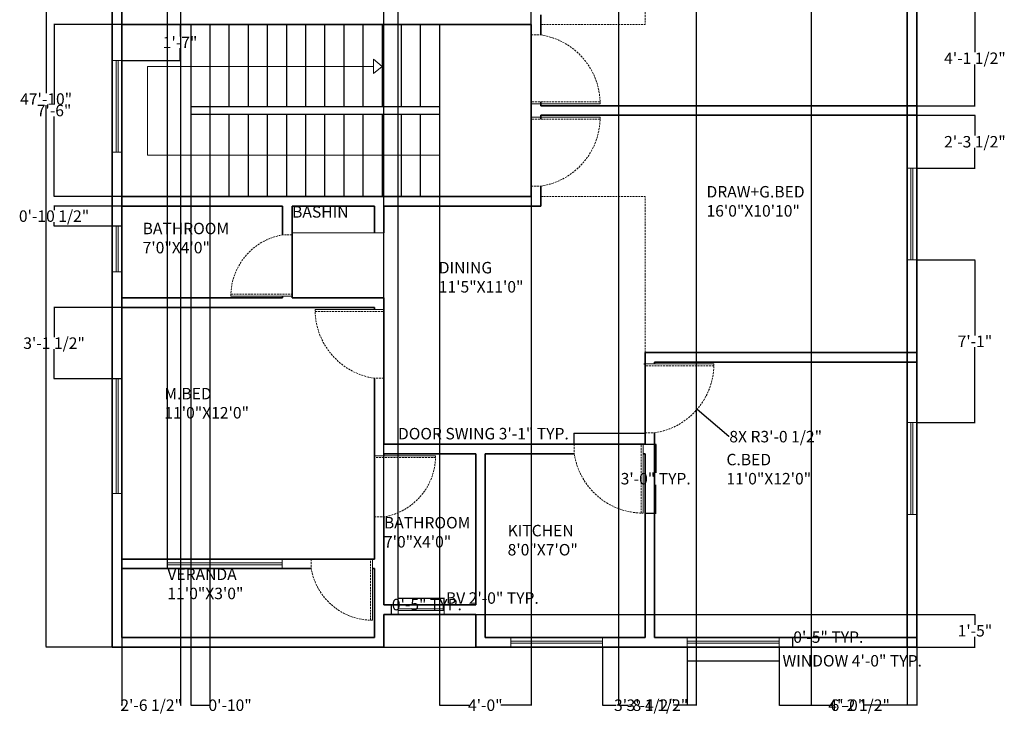
# Model space of a CAD drawing. Units: inches. Extents: x 32162 to 32679, y 109297 to 109949.
# Tile 1 of 2: x 32162 to 32677, y 109297 to 109665. Entities that reach past the tile are written whole.
import ezdxf

# ---------------------------------------------------------------- set-up
doc = ezdxf.new("R2010")
doc.units = ezdxf.units.IN
doc.header["$MEASUREMENT"] = 0
doc.linetypes.add('DASHEDX2', pattern=[1.5, 1, -0.5])
for name, color, linetype, lineweight in [('A-ANNO-DIMS', 2, 'Continuous', 18), ('A-ANNO-SYMB', 7, 'Continuous', 18), ('A-ANNO-TEXT', 7, 'Continuous', 18), ('A-AREA-BNDY', 8, 'DASHEDX2', 13), ('A-AREA-IDEN', 7, 'Continuous', 18), ('A-DOOR', 4, 'DASHEDX2', 18), ('A-FLOR-FIXT', 8, 'Continuous', 18), ('A-FLOR-STRS', 7, 'Continuous', 25), ('A-GLAZ', 30, 'Continuous', 18), ('A-WALL', 7, 'Continuous', 35)]:
    doc.layers.add(name, color=color, linetype=linetype, lineweight=lineweight)
doc.styles.get("Standard").update_dxf_attribs({"font": 'arial.ttf'})
doc.dimstyles.get("Standard").update_dxf_attribs({"dimtxt": 6, "dimasz": 0.18, "dimexe": 0.18, "dimexo": 0.0625, "dimgap": 0.09, "dimtad": 0, "dimtih": 1, "dimtoh": 1, "dimdec": 1, "dimzin": 0, "dimdsep": 46, "dimlunit": 3, "dimtxsty": 'Standard', "dimcen": 0.09, "dimadec": 0, "dimazin": 0, "dimtfac": 1, "dimtdec": 1, "dimtofl": 0, "dimtmove": 0, "dimatfit": 3, "dimfxl": 1, "dimtolj": 1, "dimtzin": 0, "dimarcsym": 0})

# ---------------------------------------------------------------- blocks, each defined once
blk = doc.blocks.new('*D2')
at = {"layer": 'A-ANNO-DIMS', "color": 0, "lineweight": -2, "transparency": 16777216}
for p, q in [((32210.5, 109909.63), (32175.8, 109909.63)), ((32175.98, 109909.45), (32175.98, 109626.28)), ((32175.98, 109336.81), (32175.98, 109619.97)), ((32210.5, 109336.63), (32175.8, 109336.63))]:
    blk.add_line(p, q, dxfattribs=at)
at = {"layer": 'A-ANNO-DIMS', "color": 0, "transparency": 16777216}
for points in [[(32175.95, 109909.45), (32176.01, 109909.45), (32175.98, 109909.63)], [(32175.95, 109336.81), (32176.01, 109336.81), (32175.98, 109336.63)]]:
    blk.add_solid(points, dxfattribs=at)
at = {"layer": 'Defpoints', "color": 0, "transparency": 16777216}
for p in [(32175.98, 109909.63), (32210.56, 109909.63), (32210.56, 109336.63)]:
    blk.add_point(p, dxfattribs=at)
at = {"layer": 'A-ANNO-DIMS', "color": 0, "transparency": 16777216, "insert": (32175.98, 109623.13), "char_height": 6, "attachment_point": 5}
blk.add_mtext('\\A1;47\'-10"', dxfattribs=at)
blk = doc.blocks.new('WIN-60IN')
for p, q in [((0, 5), (0, 0)), ((60, 5), (0, 5)), ((60, 3), (0, 3)), ((0, 2), (60, 2)), ((60, 0), (60, 5)), ((0, 0), (60, 0))]:
    blk.add_line(p, q)
blk = doc.blocks.new('BATH-VENT-24IN')
for p, q in [((0, 5), (0, 0)), ((24, 5), (0, 5)), ((24, 3), (0, 3)), ((0, 2), (24, 2)), ((24, 0), (24, 5)), ((0, 0), (24, 0))]:
    blk.add_line(p, q)
blk = doc.blocks.new('WIN-48IN')
for p, q in [((0, 5), (0, 0)), ((48, 5), (0, 5)), ((48, 3), (0, 3)), ((0, 2), (48, 2)), ((48, 0), (48, 5)), ((0, 0), (48, 0))]:
    blk.add_line(p, q)
blk = doc.blocks.new('DOOR-SWING-32IN')
for p, q in [((31, 32), (31, 0)), ((32, 0), (32, 32)), ((32, 32), (32, 0)), ((0, 0), (0, 5)), ((32, 0), (0, 0)), ((33, 0), (32, 0))]:
    blk.add_line(p, q)
blk.add_arc((32, -0.46), 32.46, 90, 170.312)
blk = doc.blocks.new('DOOR-SWING-36IN')
for p, q in [((36, 37), (31, 37)), ((36, 1), (36, 37)), ((0, 2), (36, 2)), ((36, 1), (0, 1)), ((0, 1), (36, 1)), ((36, 0), (36, 1))]:
    blk.add_line(p, q)
blk.add_arc((36.4, 1), 36.4, 98.5358, 180)
blk = doc.blocks.new('*D8')
at = {"layer": 'A-ANNO-DIMS', "color": 0, "lineweight": -2, "transparency": 16777216}
for p, q in [((32511.09, 109336.57), (32511.09, 109329.25)), ((32559.09, 109336.57), (32559.09, 109329.25)), ((32511.27, 109329.43), (32558.91, 109329.43)), ((32559.09, 109329.43), (32559.27, 109329.43))]:
    blk.add_line(p, q, dxfattribs=at)
at = {"layer": 'A-ANNO-DIMS', "color": 0, "transparency": 16777216}
for points in [[(32511.27, 109329.46), (32511.27, 109329.4), (32511.09, 109329.43)], [(32558.91, 109329.46), (32558.91, 109329.4), (32559.09, 109329.43)]]:
    blk.add_solid(points, dxfattribs=at)
at = {"layer": 'Defpoints', "color": 0, "transparency": 16777216}
for p in [(32511.09, 109336.63), (32559.09, 109336.63), (32559.09, 109329.43)]:
    blk.add_point(p, dxfattribs=at)
at = {"layer": 'A-ANNO-DIMS', "color": 0, "transparency": 16777216, "insert": (32597.33, 109329.43), "char_height": 6, "attachment_point": 5}
blk.add_mtext('\\A1;WINDOW 4\'-0" TYP.', dxfattribs=at)
blk = doc.blocks.new('*D9')
at = {"layer": 'A-ANNO-DIMS', "color": 0, "lineweight": -2, "transparency": 16777216}
for p, q in [((32559.16, 109341.63), (32566.47, 109341.63)), ((32566.29, 109341.63), (32566.29, 109341.81)), ((32566.29, 109341.81), (32566.47, 109341.81)), ((32566.29, 109336.81), (32566.29, 109341.45)), ((32559.16, 109336.63), (32566.47, 109336.63))]:
    blk.add_line(p, q, dxfattribs=at)
at = {"layer": 'A-ANNO-DIMS', "color": 0, "transparency": 16777216}
for points in [[(32566.26, 109341.45), (32566.32, 109341.45), (32566.29, 109341.63)], [(32566.26, 109336.81), (32566.32, 109336.81), (32566.29, 109336.63)]]:
    blk.add_solid(points, dxfattribs=at)
at = {"layer": 'Defpoints', "color": 0, "transparency": 16777216}
for p in [(32559.09, 109341.63), (32566.29, 109341.63), (32559.09, 109336.63)]:
    blk.add_point(p, dxfattribs=at)
at = {"layer": 'A-ANNO-DIMS', "color": 0, "transparency": 16777216, "insert": (32584.85, 109341.81), "char_height": 6, "attachment_point": 5}
blk.add_mtext('\\A1;0\'-5" TYP.', dxfattribs=at)
blk = doc.blocks.new('*D12')
at = {"layer": 'A-ANNO-DIMS', "color": 0, "lineweight": -2, "transparency": 16777216}
for p, q in [((32360.06, 109358.69), (32360.06, 109362.41)), ((32360.24, 109362.23), (32383.88, 109362.23)), ((32384.06, 109358.69), (32384.06, 109362.41)), ((32384.06, 109362.23), (32384.24, 109362.23))]:
    blk.add_line(p, q, dxfattribs=at)
at = {"layer": 'A-ANNO-DIMS', "color": 0, "transparency": 16777216}
for points in [[(32360.24, 109362.26), (32360.24, 109362.2), (32360.06, 109362.23)], [(32383.88, 109362.26), (32383.88, 109362.2), (32384.06, 109362.23)]]:
    blk.add_solid(points, dxfattribs=at)
at = {"layer": 'Defpoints', "color": 0, "transparency": 16777216}
for p in [(32384.06, 109362.23), (32360.06, 109358.63), (32384.06, 109358.63)]:
    blk.add_point(p, dxfattribs=at)
at = {"layer": 'A-ANNO-DIMS', "color": 0, "transparency": 16777216, "insert": (32409.24, 109362.23), "char_height": 6, "attachment_point": 5}
blk.add_mtext('\\A1;BV 2\'-0" TYP.', dxfattribs=at)
blk = doc.blocks.new('*D13')
at = {"layer": 'A-ANNO-DIMS', "color": 0, "lineweight": -2, "transparency": 16777216}
for p, q in [((32359.99, 109358.63), (32356.28, 109358.63)), ((32356.46, 109358.63), (32356.46, 109358.81)), ((32356.46, 109358.81), (32356.64, 109358.81)), ((32356.46, 109353.81), (32356.46, 109358.45)), ((32359.99, 109353.63), (32356.28, 109353.63))]:
    blk.add_line(p, q, dxfattribs=at)
at = {"layer": 'A-ANNO-DIMS', "color": 0, "transparency": 16777216}
for points in [[(32356.43, 109358.45), (32356.49, 109358.45), (32356.46, 109358.63)], [(32356.43, 109353.81), (32356.49, 109353.81), (32356.46, 109353.63)]]:
    blk.add_solid(points, dxfattribs=at)
at = {"layer": 'Defpoints', "color": 0, "transparency": 16777216}
for p in [(32356.46, 109358.63), (32360.06, 109358.63), (32360.06, 109353.63)]:
    blk.add_point(p, dxfattribs=at)
at = {"layer": 'A-ANNO-DIMS', "color": 0, "transparency": 16777216, "insert": (32375.01, 109358.81), "char_height": 6, "attachment_point": 5}
blk.add_mtext('\\A1;0\'-5" TYP.', dxfattribs=at)
blk = doc.blocks.new('*D14')
at = {"layer": 'A-ANNO-DIMS', "color": 0, "lineweight": -2, "transparency": 16777216}
for p, q in [((32452.06, 109448.18), (32451.88, 109448.18)), ((32452.06, 109442.69), (32452.06, 109448.36)), ((32488.88, 109448.18), (32452.24, 109448.18)), ((32489.06, 109442.69), (32489.06, 109448.36))]:
    blk.add_line(p, q, dxfattribs=at)
at = {"layer": 'A-ANNO-DIMS', "color": 0, "transparency": 16777216}
for points in [[(32452.24, 109448.21), (32452.24, 109448.15), (32452.06, 109448.18)], [(32488.88, 109448.21), (32488.88, 109448.15), (32489.06, 109448.18)]]:
    blk.add_solid(points, dxfattribs=at)
at = {"layer": 'Defpoints', "color": 0, "transparency": 16777216}
for p in [(32452.06, 109448.18), (32452.06, 109442.63), (32489.06, 109442.63)]:
    blk.add_point(p, dxfattribs=at)
at = {"layer": 'A-ANNO-DIMS', "color": 0, "transparency": 16777216, "insert": (32404.55, 109448.18), "char_height": 6, "attachment_point": 5}
blk.add_mtext('\\A1;DOOR SWING 3\'-1" TYP.', dxfattribs=at)
blk = doc.blocks.new('*D15')
at = {"layer": 'A-ANNO-DIMS', "color": 0, "lineweight": -2, "transparency": 16777216}
for p, q in [((32489.12, 109442.63), (32494.79, 109442.63)), ((32494.61, 109442.45), (32494.61, 109427.78)), ((32494.61, 109406.81), (32494.61, 109421.47)), ((32489.12, 109406.63), (32494.79, 109406.63))]:
    blk.add_line(p, q, dxfattribs=at)
at = {"layer": 'A-ANNO-DIMS', "color": 0, "transparency": 16777216}
for points in [[(32494.58, 109442.45), (32494.64, 109442.45), (32494.61, 109442.63)], [(32494.58, 109406.81), (32494.64, 109406.81), (32494.61, 109406.63)]]:
    blk.add_solid(points, dxfattribs=at)
at = {"layer": 'Defpoints', "color": 0, "transparency": 16777216}
for p in [(32489.06, 109442.63), (32494.61, 109442.63), (32489.06, 109406.63)]:
    blk.add_point(p, dxfattribs=at)
at = {"layer": 'A-ANNO-DIMS', "color": 0, "transparency": 16777216, "insert": (32494.61, 109424.63), "char_height": 6, "attachment_point": 5}
blk.add_mtext('\\A1;3\'-0" TYP.', dxfattribs=at)
blk = doc.blocks.new('*D18')
at = {"layer": 'A-ANNO-DIMS', "color": 0, "lineweight": -2, "transparency": 16777216}
for p, q in [((32215.5, 109514.13), (32179.95, 109514.13)), ((32180.13, 109513.95), (32180.13, 109498.68)), ((32180.13, 109477.03), (32180.13, 109492.3)), ((32215.5, 109476.85), (32179.95, 109476.85))]:
    blk.add_line(p, q, dxfattribs=at)
at = {"layer": 'A-ANNO-DIMS', "color": 0, "transparency": 16777216}
for points in [[(32180.1, 109513.95), (32180.16, 109513.95), (32180.13, 109514.13)], [(32180.1, 109477.03), (32180.16, 109477.03), (32180.13, 109476.85)]]:
    blk.add_solid(points, dxfattribs=at)
at = {"layer": 'Defpoints', "color": 0, "transparency": 16777216}
for p in [(32180.13, 109514.13), (32215.56, 109514.13), (32215.56, 109476.85)]:
    blk.add_point(p, dxfattribs=at)
at = {"layer": 'A-ANNO-DIMS', "color": 0, "transparency": 16777216, "insert": (32180.13, 109495.49), "char_height": 6, "attachment_point": 5}
blk.add_mtext('\\A1;3\'-1 1/2"', dxfattribs=at)
blk = doc.blocks.new('*D19')
at = {"layer": 'A-ANNO-DIMS', "color": 0, "lineweight": -2, "transparency": 16777216}
for p, q in [((32215.5, 109567.13), (32179.95, 109567.13)), ((32180.13, 109566.95), (32180.13, 109565.12)), ((32215.5, 109556.72), (32179.95, 109556.72)), ((32180.13, 109556.9), (32180.13, 109558.73))]:
    blk.add_line(p, q, dxfattribs=at)
at = {"layer": 'A-ANNO-DIMS', "color": 0, "transparency": 16777216}
for points in [[(32180.1, 109566.95), (32180.16, 109566.95), (32180.13, 109567.13)], [(32180.1, 109556.9), (32180.16, 109556.9), (32180.13, 109556.72)]]:
    blk.add_solid(points, dxfattribs=at)
at = {"layer": 'Defpoints', "color": 0, "transparency": 16777216}
for p in [(32180.13, 109567.13), (32215.56, 109567.13), (32215.56, 109556.72)]:
    blk.add_point(p, dxfattribs=at)
at = {"layer": 'A-ANNO-DIMS', "color": 0, "transparency": 16777216, "insert": (32180.13, 109561.92), "char_height": 6, "attachment_point": 5}
blk.add_mtext('\\A1;0\'-10 1/2"', dxfattribs=at)
blk = doc.blocks.new('*D20')
at = {"layer": 'A-ANNO-DIMS', "color": 0, "lineweight": -2, "transparency": 16777216}
for p, q in [((32215.62, 109662.13), (32246.17, 109662.13)), ((32245.99, 109661.95), (32245.99, 109655.85)), ((32245.99, 109643.55), (32245.99, 109649.65)), ((32215.62, 109643.37), (32246.17, 109643.37))]:
    blk.add_line(p, q, dxfattribs=at)
at = {"layer": 'A-ANNO-DIMS', "color": 0, "transparency": 16777216}
for points in [[(32245.96, 109661.95), (32246.02, 109661.95), (32245.99, 109662.13)], [(32245.96, 109643.55), (32246.02, 109643.55), (32245.99, 109643.37)]]:
    blk.add_solid(points, dxfattribs=at)
at = {"layer": 'Defpoints', "color": 0, "transparency": 16777216}
for p in [(32215.56, 109662.13), (32215.56, 109643.37), (32245.99, 109643.37)]:
    blk.add_point(p, dxfattribs=at)
at = {"layer": 'A-ANNO-DIMS', "color": 0, "transparency": 16777216, "insert": (32245.99, 109652.75), "char_height": 6, "attachment_point": 5}
blk.add_mtext('\\A1;1\'-7"', dxfattribs=at)
blk = doc.blocks.new('*D23')
at = {"layer": 'A-ANNO-DIMS', "color": 0, "lineweight": -2, "transparency": 16777216}
for p, q in [((32215.56, 109572.19), (32215.56, 109940.24)), ((32215.74, 109940.06), (32310.12, 109940.06)), ((32429.38, 109940.06), (32335.01, 109940.06)), ((32429.56, 109572.19), (32429.56, 109940.24))]:
    blk.add_line(p, q, dxfattribs=at)
at = {"layer": 'A-ANNO-DIMS', "color": 0, "transparency": 16777216}
for points in [[(32215.74, 109940.09), (32215.74, 109940.03), (32215.56, 109940.06)], [(32429.38, 109940.09), (32429.38, 109940.03), (32429.56, 109940.06)]]:
    blk.add_solid(points, dxfattribs=at)
at = {"layer": 'Defpoints', "color": 0, "transparency": 16777216}
for p in [(32429.56, 109940.06), (32215.56, 109572.13), (32429.56, 109572.13)]:
    blk.add_point(p, dxfattribs=at)
at = {"layer": 'A-ANNO-DIMS', "color": 0, "transparency": 16777216, "insert": (32322.56, 109940.06), "char_height": 6, "attachment_point": 5}
blk.add_mtext('\\A1;17\'-10"', dxfattribs=at)
blk = doc.blocks.new('*D24')
at = {"layer": 'A-ANNO-DIMS', "color": 0, "lineweight": -2, "transparency": 16777216}
for p, q in [((32215.5, 109662.13), (32179.95, 109662.13)), ((32180.13, 109661.95), (32180.13, 109620.28)), ((32180.13, 109572.31), (32180.13, 109613.97)), ((32215.5, 109572.13), (32179.95, 109572.13))]:
    blk.add_line(p, q, dxfattribs=at)
at = {"layer": 'A-ANNO-DIMS', "color": 0, "transparency": 16777216}
for points in [[(32180.1, 109661.95), (32180.16, 109661.95), (32180.13, 109662.13)], [(32180.1, 109572.31), (32180.16, 109572.31), (32180.13, 109572.13)]]:
    blk.add_solid(points, dxfattribs=at)
at = {"layer": 'Defpoints', "color": 0, "transparency": 16777216}
for p in [(32180.13, 109662.13), (32215.56, 109662.13), (32215.56, 109572.13)]:
    blk.add_point(p, dxfattribs=at)
at = {"layer": 'A-ANNO-DIMS', "color": 0, "transparency": 16777216, "insert": (32180.13, 109617.13), "char_height": 6, "attachment_point": 5}
blk.add_mtext('\\A1;7\'-6"', dxfattribs=at)
blk = doc.blocks.new('*D25')
at = {"layer": 'A-ANNO-DIMS', "color": 0, "lineweight": -2, "transparency": 16777216}
for p, q in [((32381.56, 109662.07), (32381.56, 109306.02)), ((32429.56, 109662.07), (32429.56, 109306.02)), ((32381.74, 109306.2), (32397.38, 109306.2)), ((32429.38, 109306.2), (32413.75, 109306.2))]:
    blk.add_line(p, q, dxfattribs=at)
at = {"layer": 'A-ANNO-DIMS', "color": 0, "transparency": 16777216}
for points in [[(32381.74, 109306.23), (32381.74, 109306.17), (32381.56, 109306.2)], [(32429.38, 109306.23), (32429.38, 109306.17), (32429.56, 109306.2)]]:
    blk.add_solid(points, dxfattribs=at)
at = {"layer": 'Defpoints', "color": 0, "transparency": 16777216}
for p in [(32381.56, 109662.13), (32429.56, 109662.13), (32429.56, 109306.2)]:
    blk.add_point(p, dxfattribs=at)
at = {"layer": 'A-ANNO-DIMS', "color": 0, "transparency": 16777216, "insert": (32405.56, 109306.2), "char_height": 6, "attachment_point": 5}
blk.add_mtext('\\A1;4\'-0"', dxfattribs=at)
blk = doc.blocks.new('*D26')
at = {"layer": 'A-ANNO-DIMS', "color": 0, "lineweight": -2, "transparency": 16777216}
for p, q in [((32251.56, 109662.07), (32251.56, 109306.02)), ((32261.56, 109662.07), (32261.56, 109306.02)), ((32251.74, 109306.2), (32261.38, 109306.2)), ((32261.56, 109306.2), (32261.74, 109306.2))]:
    blk.add_line(p, q, dxfattribs=at)
at = {"layer": 'A-ANNO-DIMS', "color": 0, "transparency": 16777216}
for points in [[(32251.74, 109306.23), (32251.74, 109306.17), (32251.56, 109306.2)], [(32261.38, 109306.23), (32261.38, 109306.17), (32261.56, 109306.2)]]:
    blk.add_solid(points, dxfattribs=at)
at = {"layer": 'Defpoints', "color": 0, "transparency": 16777216}
for p in [(32251.56, 109662.13), (32261.56, 109662.13), (32261.56, 109306.2)]:
    blk.add_point(p, dxfattribs=at)
at = {"layer": 'A-ANNO-DIMS', "color": 0, "transparency": 16777216, "insert": (32272.14, 109306.2), "char_height": 6, "attachment_point": 5}
blk.add_mtext('\\A1;0\'-10"', dxfattribs=at)
blk = doc.blocks.new('*D29')
at = {"layer": 'A-ANNO-DIMS', "color": 0, "lineweight": -2, "transparency": 16777216}
for p, q in [((32631.12, 109669.32), (32661.67, 109669.32)), ((32661.49, 109669.14), (32661.49, 109647.66)), ((32661.49, 109619.81), (32661.49, 109641.28)), ((32631.12, 109619.63), (32661.67, 109619.63))]:
    blk.add_line(p, q, dxfattribs=at)
at = {"layer": 'A-ANNO-DIMS', "color": 0, "transparency": 16777216}
for points in [[(32661.46, 109669.14), (32661.52, 109669.14), (32661.49, 109669.32)], [(32661.46, 109619.81), (32661.52, 109619.81), (32661.49, 109619.63)]]:
    blk.add_solid(points, dxfattribs=at)
at = {"layer": 'Defpoints', "color": 0, "transparency": 16777216}
for p in [(32631.06, 109669.32), (32631.06, 109619.63), (32661.49, 109619.63)]:
    blk.add_point(p, dxfattribs=at)
at = {"layer": 'A-ANNO-DIMS', "color": 0, "transparency": 16777216, "insert": (32661.49, 109644.47), "char_height": 6, "attachment_point": 5}
blk.add_mtext('\\A1;4\'-1 1/2"', dxfattribs=at)
blk = doc.blocks.new('*D30')
at = {"layer": 'A-ANNO-DIMS', "color": 0, "lineweight": -2, "transparency": 16777216}
for p, q in [((32631.12, 109614.63), (32661.67, 109614.63)), ((32661.49, 109614.45), (32661.49, 109604)), ((32661.49, 109587.16), (32661.49, 109597.61)), ((32631.12, 109586.98), (32661.67, 109586.98))]:
    blk.add_line(p, q, dxfattribs=at)
at = {"layer": 'A-ANNO-DIMS', "color": 0, "transparency": 16777216}
for points in [[(32661.46, 109614.45), (32661.52, 109614.45), (32661.49, 109614.63)], [(32661.46, 109587.16), (32661.52, 109587.16), (32661.49, 109586.98)]]:
    blk.add_solid(points, dxfattribs=at)
at = {"layer": 'Defpoints', "color": 0, "transparency": 16777216}
for p in [(32631.06, 109614.63), (32631.06, 109586.98), (32661.49, 109586.98)]:
    blk.add_point(p, dxfattribs=at)
at = {"layer": 'A-ANNO-DIMS', "color": 0, "transparency": 16777216, "insert": (32661.49, 109600.8), "char_height": 6, "attachment_point": 5}
blk.add_mtext('\\A1;2\'-3 1/2"', dxfattribs=at)
blk = doc.blocks.new('*D31')
at = {"layer": 'A-ANNO-DIMS', "color": 0, "lineweight": -2, "transparency": 16777216}
for p, q in [((32631.12, 109538.98), (32661.67, 109538.98)), ((32661.49, 109538.8), (32661.49, 109499.57)), ((32661.49, 109454.15), (32661.49, 109493.37)), ((32631.12, 109453.97), (32661.67, 109453.97))]:
    blk.add_line(p, q, dxfattribs=at)
at = {"layer": 'A-ANNO-DIMS', "color": 0, "transparency": 16777216}
for points in [[(32661.46, 109538.8), (32661.52, 109538.8), (32661.49, 109538.98)], [(32661.46, 109454.15), (32661.52, 109454.15), (32661.49, 109453.97)]]:
    blk.add_solid(points, dxfattribs=at)
at = {"layer": 'Defpoints', "color": 0, "transparency": 16777216}
for p in [(32631.06, 109538.98), (32631.06, 109453.97), (32661.49, 109453.97)]:
    blk.add_point(p, dxfattribs=at)
at = {"layer": 'A-ANNO-DIMS', "color": 0, "transparency": 16777216, "insert": (32661.49, 109496.47), "char_height": 6, "attachment_point": 5}
blk.add_mtext('\\A1;7\'-1"', dxfattribs=at)
blk = doc.blocks.new('*D32')
at = {"layer": 'A-ANNO-DIMS', "color": 0, "lineweight": -2, "transparency": 16777216}
for p, q in [((32475.17, 109904.57), (32475.17, 109306.02)), ((32515.81, 109904.57), (32515.81, 109306.02)), ((32475.35, 109306.2), (32480.44, 109306.2)), ((32515.63, 109306.2), (32510.54, 109306.2))]:
    blk.add_line(p, q, dxfattribs=at)
at = {"layer": 'A-ANNO-DIMS', "color": 0, "transparency": 16777216}
for points in [[(32475.35, 109306.23), (32475.35, 109306.17), (32475.17, 109306.2)], [(32515.63, 109306.23), (32515.63, 109306.17), (32515.81, 109306.2)]]:
    blk.add_solid(points, dxfattribs=at)
at = {"layer": 'Defpoints', "color": 0, "transparency": 16777216}
for p in [(32475.17, 109904.63), (32515.81, 109904.63), (32515.81, 109306.2)]:
    blk.add_point(p, dxfattribs=at)
at = {"layer": 'A-ANNO-DIMS', "color": 0, "transparency": 16777216, "insert": (32495.49, 109306.2), "char_height": 6, "attachment_point": 5}
blk.add_mtext('\\A1;3\'-4 1/2"', dxfattribs=at)
blk = doc.blocks.new('*D33')
at = {"layer": 'A-ANNO-DIMS', "color": 0, "lineweight": -2, "transparency": 16777216}
for p, q in [((32575.81, 109904.57), (32575.81, 109306.02)), ((32626.06, 109904.57), (32626.06, 109306.02)), ((32575.99, 109306.2), (32585.76, 109306.2)), ((32625.88, 109306.2), (32616.11, 109306.2))]:
    blk.add_line(p, q, dxfattribs=at)
at = {"layer": 'A-ANNO-DIMS', "color": 0, "transparency": 16777216}
for points in [[(32575.99, 109306.23), (32575.99, 109306.17), (32575.81, 109306.2)], [(32625.88, 109306.23), (32625.88, 109306.17), (32626.06, 109306.2)]]:
    blk.add_solid(points, dxfattribs=at)
at = {"layer": 'Defpoints', "color": 0, "transparency": 16777216}
for p in [(32575.81, 109904.63), (32626.06, 109904.63), (32626.06, 109306.2)]:
    blk.add_point(p, dxfattribs=at)
at = {"layer": 'A-ANNO-DIMS', "color": 0, "transparency": 16777216, "insert": (32600.94, 109306.2), "char_height": 6, "attachment_point": 5}
blk.add_mtext('\\A1;4\'-2 1/2"', dxfattribs=at)
blk = doc.blocks.new('*D34')
at = {"layer": 'A-ANNO-DIMS', "color": 0, "lineweight": -2, "transparency": 16777216}
for p, q in [((32466.82, 109336.57), (32466.82, 109306.02)), ((32511.09, 109336.57), (32511.09, 109306.02)), ((32467, 109306.2), (32473.9, 109306.2)), ((32510.91, 109306.2), (32504.01, 109306.2))]:
    blk.add_line(p, q, dxfattribs=at)
at = {"layer": 'A-ANNO-DIMS', "color": 0, "transparency": 16777216}
for points in [[(32467, 109306.23), (32467, 109306.17), (32466.82, 109306.2)], [(32510.91, 109306.23), (32510.91, 109306.17), (32511.09, 109306.2)]]:
    blk.add_solid(points, dxfattribs=at)
at = {"layer": 'Defpoints', "color": 0, "transparency": 16777216}
for p in [(32466.82, 109336.63), (32511.09, 109336.63), (32511.09, 109306.2)]:
    blk.add_point(p, dxfattribs=at)
at = {"layer": 'A-ANNO-DIMS', "color": 0, "transparency": 16777216, "insert": (32488.96, 109306.2), "char_height": 6, "attachment_point": 5}
blk.add_mtext('\\A1;3\'-8 1/2"', dxfattribs=at)
blk = doc.blocks.new('*D35')
at = {"layer": 'A-ANNO-DIMS', "color": 0, "lineweight": -2, "transparency": 16777216}
for p, q in [((32559.09, 109336.57), (32559.09, 109306.02)), ((32631.06, 109336.57), (32631.06, 109306.02)), ((32559.27, 109306.2), (32587, 109306.2)), ((32630.88, 109306.2), (32603.16, 109306.2))]:
    blk.add_line(p, q, dxfattribs=at)
at = {"layer": 'A-ANNO-DIMS', "color": 0, "transparency": 16777216}
for points in [[(32559.27, 109306.23), (32559.27, 109306.17), (32559.09, 109306.2)], [(32630.88, 109306.23), (32630.88, 109306.17), (32631.06, 109306.2)]]:
    blk.add_solid(points, dxfattribs=at)
at = {"layer": 'Defpoints', "color": 0, "transparency": 16777216}
for p in [(32559.09, 109336.63), (32631.06, 109336.63), (32631.06, 109306.2)]:
    blk.add_point(p, dxfattribs=at)
at = {"layer": 'A-ANNO-DIMS', "color": 0, "transparency": 16777216, "insert": (32595.08, 109306.2), "char_height": 6, "attachment_point": 5}
blk.add_mtext('\\A1;6\'-0"', dxfattribs=at)
blk = doc.blocks.new('*D37')
at = {"layer": 'A-ANNO-DIMS', "color": 0, "lineweight": -2, "transparency": 16777216}
for p, q in [((32352.62, 109353.63), (32661.67, 109353.63)), ((32661.49, 109353.45), (32661.49, 109348.28)), ((32661.49, 109336.81), (32661.49, 109341.97)), ((32352.62, 109336.63), (32661.67, 109336.63))]:
    blk.add_line(p, q, dxfattribs=at)
at = {"layer": 'A-ANNO-DIMS', "color": 0, "transparency": 16777216}
for points in [[(32661.46, 109353.45), (32661.52, 109353.45), (32661.49, 109353.63)], [(32661.46, 109336.81), (32661.52, 109336.81), (32661.49, 109336.63)]]:
    blk.add_solid(points, dxfattribs=at)
at = {"layer": 'Defpoints', "color": 0, "transparency": 16777216}
for p in [(32352.56, 109353.63), (32661.49, 109353.63), (32352.56, 109336.63)]:
    blk.add_point(p, dxfattribs=at)
at = {"layer": 'A-ANNO-DIMS', "color": 0, "transparency": 16777216, "insert": (32661.49, 109345.13), "char_height": 6, "attachment_point": 5}
blk.add_mtext('\\A1;1\'-5"', dxfattribs=at)
blk = doc.blocks.new('*D39')
at = {"layer": 'A-ANNO-DIMS', "color": 0, "lineweight": -2, "transparency": 16777216}
for p, q in [((32352.56, 109358.69), (32352.56, 109940.24)), ((32352.74, 109940.06), (32359.88, 109940.06)), ((32360.06, 109358.69), (32360.06, 109940.24)), ((32360.06, 109940.06), (32360.24, 109940.06))]:
    blk.add_line(p, q, dxfattribs=at)
at = {"layer": 'A-ANNO-DIMS', "color": 0, "transparency": 16777216}
for points in [[(32352.74, 109940.09), (32352.74, 109940.03), (32352.56, 109940.06)], [(32359.88, 109940.09), (32359.88, 109940.03), (32360.06, 109940.06)]]:
    blk.add_solid(points, dxfattribs=at)
at = {"layer": 'Defpoints', "color": 0, "transparency": 16777216}
for p in [(32360.06, 109940.06), (32352.56, 109358.63), (32360.06, 109358.63)]:
    blk.add_point(p, dxfattribs=at)
at = {"layer": 'A-ANNO-DIMS', "color": 0, "transparency": 16777216, "insert": (32375.29, 109940.06), "char_height": 6, "attachment_point": 5}
blk.add_mtext('\\A1;0\'-7 1/2"', dxfattribs=at)
blk = doc.blocks.new('*D40')
at = {"layer": 'A-ANNO-DIMS', "color": 0, "lineweight": -2, "transparency": 16777216}
for p, q in [((32215.561139, 109863.565361), (32215.561139, 109306.020361)), ((32246.241611, 109863.565361), (32246.241611, 109306.020361)), ((32215.381139, 109306.200361), (32215.201139, 109306.200361)), ((32246.421611, 109306.200361), (32246.601611, 109306.200361))]:
    blk.add_line(p, q, dxfattribs=at)
at = {"layer": 'A-ANNO-DIMS', "color": 0, "transparency": 16777216}
for points in [[(32215.381139, 109306.230361), (32215.381139, 109306.170361), (32215.561139, 109306.200361)], [(32246.421611, 109306.230361), (32246.421611, 109306.170361), (32246.241611, 109306.200361)]]:
    blk.add_solid(points, dxfattribs=at)
at = {"layer": 'Defpoints', "color": 0, "transparency": 16777216}
for p in [(32215.561139, 109863.627861), (32246.241611, 109863.627861), (32246.241611, 109306.200361)]:
    blk.add_point(p, dxfattribs=at)
at = {"layer": 'A-ANNO-DIMS', "color": 0, "transparency": 16777216, "insert": (32230.901375, 109306.200361), "char_height": 6, "attachment_point": 5}
blk.add_mtext('\\A1;2\'-6 1/2"', dxfattribs=at)
blk = doc.blocks.new('*D41')
at = {"layer": 'A-ANNO-DIMS', "color": 0, "lineweight": -2, "transparency": 16777216}
for p, q in [((32215.56, 109377.69), (32215.56, 109940.24)), ((32215.74, 109940.06), (32219.36, 109940.06)), ((32239.21, 109940.06), (32235.59, 109940.06)), ((32239.39, 109377.69), (32239.39, 109940.24))]:
    blk.add_line(p, q, dxfattribs=at)
at = {"layer": 'A-ANNO-DIMS', "color": 0, "transparency": 16777216}
for points in [[(32215.74, 109940.09), (32215.74, 109940.03), (32215.56, 109940.06)], [(32239.21, 109940.09), (32239.21, 109940.03), (32239.39, 109940.06)]]:
    blk.add_solid(points, dxfattribs=at)
at = {"layer": 'Defpoints', "color": 0, "transparency": 16777216}
for p in [(32239.39, 109940.06), (32215.56, 109377.63), (32239.39, 109377.63)]:
    blk.add_point(p, dxfattribs=at)
at = {"layer": 'A-ANNO-DIMS', "color": 0, "transparency": 16777216, "insert": (32227.48, 109940.06), "char_height": 6, "attachment_point": 5}
blk.add_mtext('\\A1;2\'-0"', dxfattribs=at)
blk = doc.blocks.new('*D42')
at = {"layer": 'A-ANNO-DIMS', "color": 0, "lineweight": -2, "transparency": 16777216}
for p, q in [((32488.57, 109484.63), (32488.75, 109484.63)), ((32488.66, 109484.54), (32488.66, 109484.72)), ((32532.79, 109446.62), (32516.38, 109460.76)), ((32532.97, 109446.62), (32532.79, 109446.62))]:
    blk.add_line(p, q, dxfattribs=at)
at = {"layer": 'A-ANNO-DIMS', "color": 0, "transparency": 16777216}
blk.add_solid([(32516.4, 109460.78), (32516.36, 109460.73), (32516.24, 109460.87)], dxfattribs=at)
at = {"layer": 'Defpoints', "color": 0, "transparency": 16777216}
for p in [(32488.66, 109484.63), (32516.24, 109460.87)]:
    blk.add_point(p, dxfattribs=at)
at = {"layer": 'A-ANNO-DIMS', "color": 0, "transparency": 16777216, "insert": (32557.35, 109446.62), "char_height": 6, "attachment_point": 5}
blk.add_mtext('\\A1;8X R3\'-0 1/2"', dxfattribs=at)

msp = doc.modelspace()

# ---------------------------------------------------------------- linework, layer by layer
at = {"layer": 'A-ANNO-SYMB'}
for p, q in [((32351.56, 109640.17), (32347.08, 109643.93)), ((32347.08, 109643.93), (32347.08, 109636.41)), ((32228.93, 109593.75), (32228.93, 109640.17)), ((32228.93, 109640.17), (32347.08, 109640.17)), ((32351.56, 109640.17), (32347.08, 109636.41)), ((32381.56, 109593.75), (32228.93, 109593.75))]:
    msp.add_line(p, q, dxfattribs=at)
at = {"layer": 'A-AREA-BNDY'}
for p, q in [((32489.06, 109755.63), (32489.06, 109662.13)), ((32434.56, 109662.13), (32489.06, 109662.13)), ((32434.56, 109572.13), (32489.06, 109572.13)), ((32489.06, 109490.63), (32489.06, 109572.13))]:
    msp.add_line(p, q, dxfattribs=at)
at = {"layer": 'A-FLOR-FIXT'}
msp.add_line((32304.56, 109553.24), (32352.56, 109553.24), dxfattribs=at)
at = {"layer": 'A-FLOR-STRS'}
for p, q in [((32215.56, 109662.13), (32251.56, 109662.13)), ((32251.56, 109662.13), (32251.56, 109572.13)), ((32261.56, 109662.13), (32261.56, 109619.13)), ((32271.56, 109662.13), (32271.56, 109619.13)), ((32281.56, 109662.13), (32281.56, 109619.13)), ((32291.56, 109662.13), (32291.56, 109619.13)), ((32301.56, 109662.13), (32301.56, 109619.13)), ((32311.56, 109662.13), (32311.56, 109619.13)), ((32321.56, 109662.13), (32321.56, 109619.13)), ((32331.56, 109662.13), (32331.56, 109619.13)), ((32341.56, 109662.13), (32341.56, 109619.13)), ((32351.56, 109662.13), (32351.56, 109619.13)), ((32361.56, 109662.13), (32361.56, 109619.13)), ((32371.56, 109662.13), (32371.56, 109619.13)), ((32381.56, 109662.13), (32381.56, 109572.13)), ((32381.56, 109619.13), (32251.56, 109619.13)), ((32381.56, 109615.13), (32251.56, 109615.13)), ((32261.56, 109615.13), (32261.56, 109572.13)), ((32271.56, 109615.13), (32271.56, 109572.13)), ((32281.56, 109615.13), (32281.56, 109572.13)), ((32291.56, 109615.13), (32291.56, 109572.13)), ((32301.56, 109615.13), (32301.56, 109572.13)), ((32311.56, 109615.13), (32311.56, 109572.13)), ((32321.56, 109615.13), (32321.56, 109572.13)), ((32331.56, 109615.13), (32331.56, 109572.13)), ((32341.56, 109615.13), (32341.56, 109572.13)), ((32351.56, 109615.13), (32351.56, 109572.13)), ((32361.56, 109615.13), (32361.56, 109572.13)), ((32371.56, 109615.13), (32371.56, 109572.13))]:
    msp.add_line(p, q, dxfattribs=at)
at = {"layer": 'A-GLAZ'}
for p, q in [((32210.56, 109416.85), (32210.56, 109416.85)), ((32418.82, 109341.63), (32418.82, 109341.63)), ((32511.09, 109341.63), (32511.09, 109341.63)), ((32418.82, 109336.63), (32418.82, 109336.63))]:
    msp.add_line(p, q, dxfattribs=at)
at = {"layer": 'A-WALL'}
for p, q in [((32210.56, 109909.63), (32210.56, 109662.13)), ((32631.06, 109909.63), (32631.06, 109336.63)), ((32626.06, 109755.63), (32626.06, 109336.63)), ((32434.56, 109667.13), (32434.56, 109656.63)), ((32210.56, 109662.13), (32210.56, 109643.37)), ((32215.56, 109662.13), (32429.56, 109662.13)), ((32215.56, 109662.13), (32215.56, 109643.37)), ((32429.56, 109662.13), (32429.56, 109572.13)), ((32429.56, 109662.13), (32429.56, 109572.13)), ((32210.56, 109643.37), (32210.56, 109336.63)), ((32215.56, 109643.37), (32215.56, 109572.13)), ((32429.56, 109572.13), (32429.56, 109617.13)), ((32434.56, 109621.63), (32434.56, 109619.63)), ((32434.56, 109619.63), (32631.06, 109619.63)), ((32434.56, 109614.63), (32631.06, 109614.63)), ((32434.56, 109614.63), (32434.56, 109612.63)), ((32434.56, 109577.63), (32434.56, 109567.13)), ((32215.56, 109572.13), (32429.56, 109572.13)), ((32215.56, 109567.13), (32299.56, 109567.13)), ((32215.56, 109567.13), (32215.56, 109519.13)), ((32299.56, 109567.13), (32299.56, 109552.13)), ((32299.56, 109567.13), (32299.56, 109552.13)), ((32304.56, 109567.13), (32304.56, 109519.13)), ((32304.56, 109567.13), (32347.56, 109567.13)), ((32347.56, 109567.13), (32347.56, 109553.24)), ((32352.56, 109567.13), (32352.56, 109553.24)), ((32352.56, 109567.13), (32434.56, 109567.13)), ((32352.56, 109548.13), (32352.56, 109548.13)), ((32299.56, 109520.13), (32299.56, 109519.13)), ((32215.56, 109519.13), (32299.56, 109519.13)), ((32215.56, 109514.13), (32347.56, 109514.13)), ((32215.56, 109514.13), (32215.56, 109382.63)), ((32304.56, 109519.13), (32352.56, 109519.13)), ((32347.56, 109514.13), (32347.56, 109513.13)), ((32352.56, 109519.13), (32352.56, 109442.63)), ((32489.06, 109490.63), (32631.06, 109490.63)), ((32489.06, 109490.63), (32489.06, 109442.63)), ((32494.06, 109485.63), (32631.06, 109485.63)), ((32494.06, 109485.63), (32494.06, 109484.63)), ((32347.56, 109477.13), (32347.56, 109382.63)), ((32494.06, 109448.63), (32494.06, 109341.63)), ((32352.56, 109442.63), (32489.06, 109442.63)), ((32352.56, 109437.63), (32400.56, 109437.63)), ((32352.56, 109437.63), (32352.56, 109436.63)), ((32400.56, 109437.63), (32400.56, 109358.63)), ((32405.56, 109437.63), (32405.56, 109341.63)), ((32405.56, 109437.63), (32452.06, 109437.63)), ((32488.06, 109437.63), (32489.06, 109437.63)), ((32489.06, 109437.63), (32489.06, 109341.63)), ((32352.56, 109404.63), (32352.56, 109358.63)), ((32215.56, 109382.63), (32347.56, 109382.63)), ((32215.56, 109377.63), (32314.56, 109377.63)), ((32215.56, 109377.63), (32215.56, 109341.63)), ((32346.56, 109377.63), (32347.56, 109377.63)), ((32347.56, 109377.63), (32347.56, 109341.63)), ((32352.56, 109358.63), (32400.56, 109358.63)), ((32352.56, 109353.63), (32400.56, 109353.63)), ((32352.56, 109353.63), (32352.56, 109336.63)), ((32400.56, 109353.63), (32400.56, 109336.63)), ((32215.56, 109341.63), (32347.56, 109341.63)), ((32405.56, 109341.63), (32489.06, 109341.63)), ((32494.06, 109341.63), (32631.06, 109341.63)), ((32210.56, 109336.63), (32352.56, 109336.63)), ((32400.56, 109336.63), (32631.06, 109336.63))]:
    msp.add_line(p, q, dxfattribs=at)

# ---------------------------------------------------------------- block references
at = {"layer": 'A-DOOR', "extrusion": (0, 0, -1), "zscale": -1}
msp.add_blockref('DOOR-SWING-36IN', (-32465.56, 109619.63), dxfattribs=at)
at = {"layer": 'A-DOOR'}
for p, rotation in [((32465.56, 109614.63), 180), ((32525.06, 109485.63), 180), ((32489.06, 109406.63), 89.99999999998359)]:
    msp.add_blockref('DOOR-SWING-36IN', p, dxfattribs=dict(at, rotation=rotation))
at = {"layer": 'A-DOOR', "extrusion": (0, 0, -1), "zscale": -1}
for name, p, rotation in [('DOOR-SWING-32IN', (-32304.56, 109552.13), 269.9999999999738), ('DOOR-SWING-36IN', (-32316.56, 109514.13), 180), ('DOOR-SWING-32IN', (-32347.56, 109404.63), 89.99999999994625), ('DOOR-SWING-32IN', (-32314.56, 109382.63), 180)]:
    msp.add_blockref(name, p, dxfattribs=dict(at, rotation=rotation))
at = {"layer": 'A-GLAZ'}
for name, p, rotation in [('WIN-48IN', (32210.56, 109643.37), 270.000000000042), ('WIN-48IN', (32626.06, 109586.98), 270.0000000000163), ('BATH-VENT-24IN', (32210.56, 109556.72), 270.0000000000833), ('WIN-60IN', (32210.56, 109476.85), 270.0000000000149), ('WIN-48IN', (32626.06, 109453.97), 270.0000000000091)]:
    msp.add_blockref(name, p, dxfattribs=dict(at, rotation=rotation))
for name, p in [('WIN-60IN', (32239.39, 109377.63)), ('BATH-VENT-24IN', (32360.06, 109353.63)), ('WIN-48IN', (32418.82, 109336.63)), ('WIN-48IN', (32511.09, 109336.63))]:
    msp.add_blockref(name, p, dxfattribs=at)

# ---------------------------------------------------------------- texts
at = {"layer": 'A-ANNO-TEXT', "insert": (32304.56, 109567.13), "char_height": 6, "attachment_point": 1}
msp.add_mtext_dynamic_manual_height_columns('BASHIN', width=43, gutter_width=30, heights=[0], dxfattribs=at)
at = {"layer": 'A-AREA-IDEN', "char_height": 6, "attachment_point": 1}
for s, width, insert in [('DRAW+G.BED\\P16\'0"X10\'10"', 82.1998, (32521.18, 109577.66)), ('BATHROOM\\P7\'0"X4\'0"', 53.7787, (32226.43, 109558.45)), ('DINING\\P11\'5"X11\'0"', 93.6329, (32381.23, 109537.97)), ('M.BED\\P11\'0"X12\'0"', 98.9924, (32237.78, 109472.1)), ('C.BED\\P11\'0"X12\'0"', 70.6187, (32531.61, 109437.63)), ('BATHROOM \\P7\'0"X4\'0"', 26.13, (32352.56, 109404.63)), ('KITCHEN\\P8\'0"X7\'O"', 55.6014, (32417.22, 109400.49)), ('VERANDA\\P11\'0"X3\'0"', 60.182, (32239.39, 109377.63))]:
    msp.add_mtext_dynamic_manual_height_columns(s, width=width, gutter_width=30, heights=[0], dxfattribs=dict(at, insert=insert))

# ---------------------------------------------------------------- dimensions: what is measured, and where the dimension line sits
at = {"layer": 'A-ANNO-DIMS'}
for base, p1, p2, picture, middle in [((32360.06, 109940.06), (32352.56, 109358.63), (32360.06, 109358.63), '*D39', (32375.29, 109940.06)), ((32429.56, 109940.06), (32215.56, 109572.13), (32429.56, 109572.13), '*D23', (32322.56, 109940.06)), ((32239.39, 109940.06), (32215.56, 109377.63), (32239.39, 109377.63), '*D41', (32227.48, 109940.06)), ((32515.81, 109306.2), (32475.17, 109904.63), (32515.81, 109904.63), '*D32', (32495.49, 109306.2)), ((32626.061139, 109306.200361), (32575.811139, 109904.627861), (32626.061139, 109904.627861), '*D33', (32600.936139, 109306.200361)), ((32246.24, 109306.2), (32215.56, 109863.63), (32246.24, 109863.63), '*D40', (32230.9, 109306.2)), ((32261.56, 109306.2), (32251.56, 109662.13), (32261.56, 109662.13), '*D26', (32272.14, 109306.2)), ((32429.56, 109306.2), (32381.56, 109662.13), (32429.56, 109662.13), '*D25', (32405.56, 109306.2)), ((32511.09, 109306.2), (32466.82, 109336.63), (32511.09, 109336.63), '*D34', (32488.96, 109306.2)), ((32631.06, 109306.2), (32559.09, 109336.63), (32631.06, 109336.63), '*D35', (32595.08, 109306.2))]:
    dim = msp.add_linear_dim(base=base, p1=p1, p2=p2, dimstyle='Standard', override={"dimdec": 1, "dimlfac": 1, "dimrnd": 0, "dimzin": 1, "dimdsep": 46, "dimlunit": 4, "dimfrac": 2}, dxfattribs=at)
    dim.commit()
    dim.dimension.update_dxf_attribs({"geometry": picture, "text_midpoint": middle})
for base, p1, p2, angle, text, override, picture, middle in [((32175.98, 109909.63), (32210.56, 109336.63), (32210.56, 109909.63), 90, '47\'-10"', {"dimclrd": 0, "dimclre": 0, "dimclrt": 0}, '*D2', (32175.98, 109623.13)), ((32452.06, 109448.18), (32489.06, 109442.63), (32452.06, 109442.63), 180, 'DOOR SWING <> TYP.', {"dimdec": 1, "dimlfac": 1, "dimrnd": 0, "dimzin": 1, "dimdsep": 46, "dimlunit": 4, "dimfrac": 2}, '*D14', (32404.55, 109448.18)), ((32494.61, 109442.63), (32489.06, 109406.63), (32489.06, 109442.63), 90, '<> TYP.', {"dimdec": 1, "dimlfac": 1, "dimrnd": 0, "dimzin": 1, "dimdsep": 46, "dimlunit": 4, "dimfrac": 2}, '*D15', (32494.61, 109424.63)), ((32356.46, 109358.63), (32360.06, 109353.63), (32360.06, 109358.63), 90, '<> TYP.', {"dimdec": 1, "dimlfac": 1, "dimrnd": 0, "dimzin": 1, "dimdsep": 46, "dimlunit": 4, "dimfrac": 2}, '*D13', (32375.01, 109358.81)), ((32566.29, 109341.63), (32559.09, 109336.63), (32559.09, 109341.63), 90, '<> TYP.', {"dimdec": 1, "dimlfac": 1, "dimrnd": 0, "dimzin": 1, "dimdsep": 46, "dimlunit": 4, "dimfrac": 2}, '*D9', (32584.85, 109341.81))]:
    dim = msp.add_linear_dim(base=base, p1=p1, p2=p2, angle=angle, text=text, dimstyle='Standard', override=override, dxfattribs=at)
    dim.commit()
    dim.dimension.update_dxf_attribs({"geometry": picture, "text_midpoint": middle})
for base, p1, p2, angle, picture, middle in [((32661.49, 109619.63), (32631.06, 109669.32), (32631.06, 109619.63), 90, '*D29', (32661.49, 109644.47)), ((32180.13, 109662.13), (32215.56, 109572.13), (32215.56, 109662.13), 90, '*D24', (32180.13, 109617.13)), ((32245.99, 109643.37), (32215.56, 109662.13), (32215.56, 109643.37), 270, '*D20', (32245.99, 109652.75)), ((32661.4886, 109586.9765), (32631.0611, 109614.6279), (32631.0611, 109586.9765), 90, '*D30', (32661.4886, 109600.8022)), ((32180.13, 109567.13), (32215.56, 109556.72), (32215.56, 109567.13), 90, '*D19', (32180.13, 109561.92)), ((32661.49, 109453.97), (32631.06, 109538.98), (32631.06, 109453.97), 90, '*D31', (32661.49, 109496.47)), ((32180.13, 109514.13), (32215.56, 109476.85), (32215.56, 109514.13), 90, '*D18', (32180.13, 109495.49)), ((32661.49, 109353.63), (32352.56, 109336.63), (32352.56, 109353.63), 90, '*D37', (32661.49, 109345.13))]:
    dim = msp.add_linear_dim(base=base, p1=p1, p2=p2, angle=angle, dimstyle='Standard', override={"dimdec": 1, "dimlfac": 1, "dimrnd": 0, "dimzin": 1, "dimdsep": 46, "dimlunit": 4, "dimfrac": 2}, dxfattribs=at)
    dim.commit()
    dim.dimension.update_dxf_attribs({"geometry": picture, "text_midpoint": middle})
dim = msp.add_radius_dim(center=(32488.66, 109484.63), mpoint=(32516.24, 109460.87), text='8X <>', dimstyle='Standard', override={"dimdec": 1, "dimlfac": 1, "dimrnd": 0, "dimzin": 1, "dimdsep": 46, "dimlunit": 4, "dimfrac": 2}, dxfattribs=at)
dim.commit()
dim.dimension.update_dxf_attribs({"geometry": '*D42', "text_midpoint": (32557.35, 109446.62), "dimtype": 164})
for base, p1, p2, text, picture, middle in [((32384.06, 109362.23), (32360.06, 109358.63), (32384.06, 109358.63), 'BV <> TYP.', '*D12', (32409.24, 109362.23)), ((32559.09, 109329.43), (32511.09, 109336.63), (32559.09, 109336.63), 'WINDOW <> TYP.', '*D8', (32597.33, 109329.43))]:
    dim = msp.add_linear_dim(base=base, p1=p1, p2=p2, text=text, dimstyle='Standard', override={"dimdec": 1, "dimlfac": 1, "dimrnd": 0, "dimzin": 1, "dimdsep": 46, "dimlunit": 4, "dimfrac": 2}, dxfattribs=at)
    dim.commit()
    dim.dimension.update_dxf_attribs({"geometry": picture, "text_midpoint": middle})

doc.saveas('drawing.dxf')
